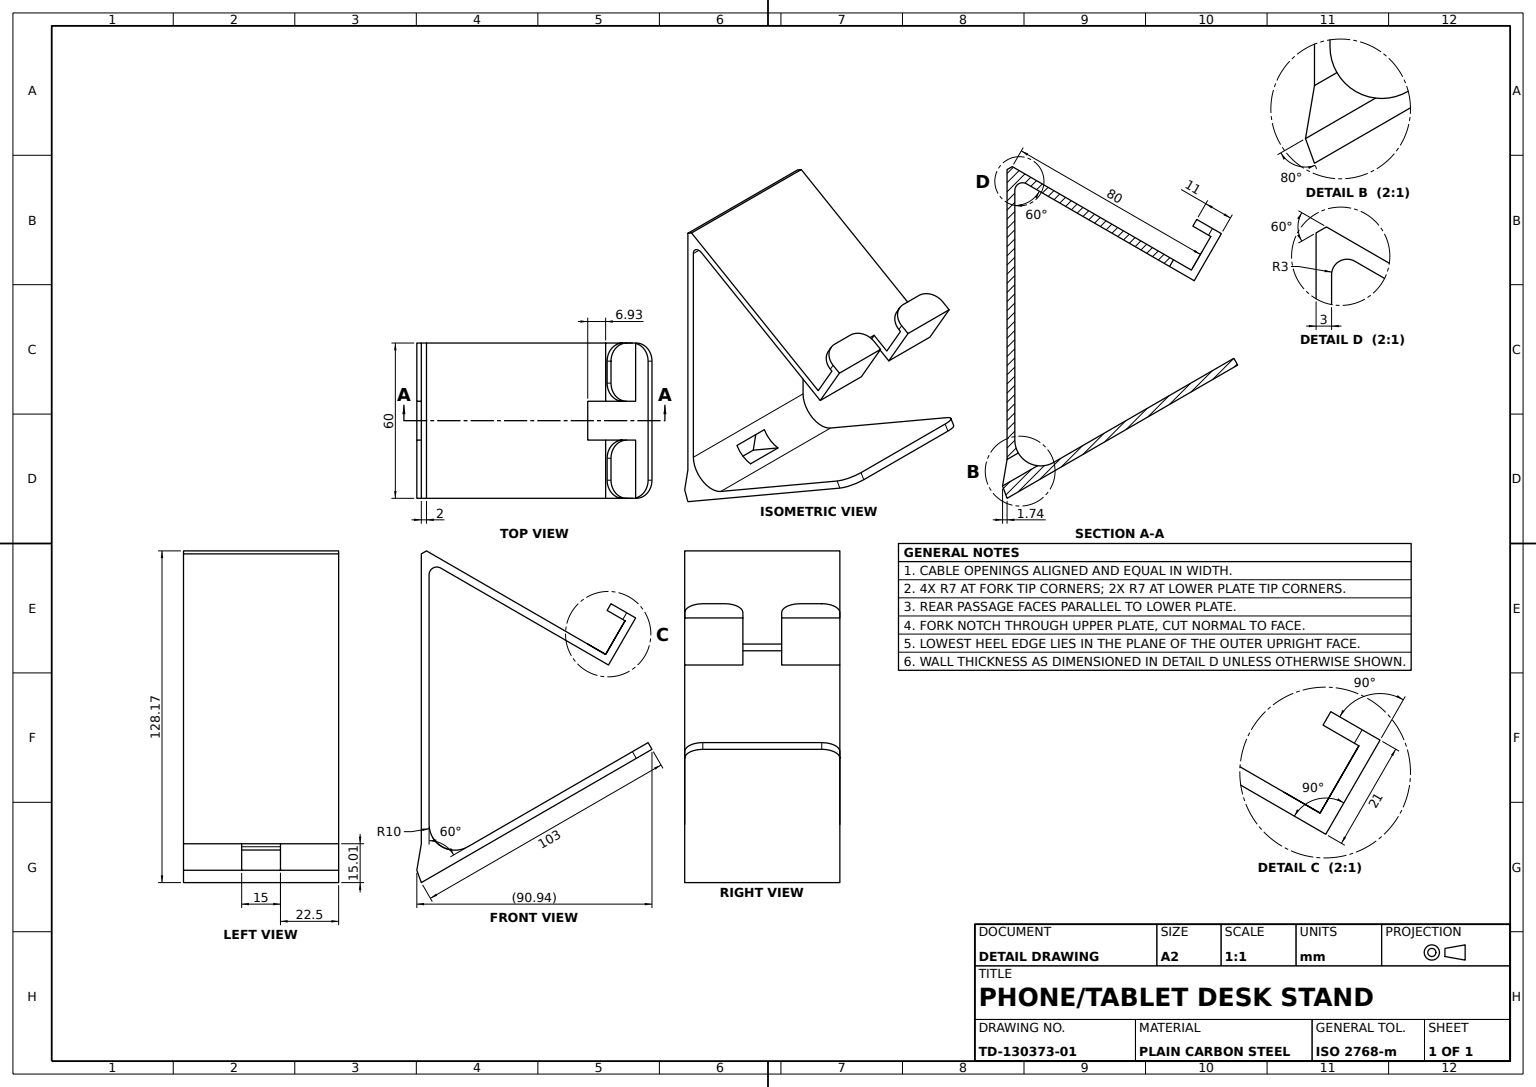
from build123d import *

# Parameters (mm, degrees)
STAND_BODY_60MM_DEPTH = 30
CABLE_NOTCH_SKETCH_W  = 15
CABLE_NOTCH_SKETCH_H  = 8
CABLE_NOTCH_DEPTH     = 152.518975709
SLOT_15X11_REACH      = 167.253
SLOT_15X11_SKETCH_W   = 15
SLOT_15X11_SKETCH_H   = 11
SLOT_EDGE_FILLET_R7_R = 7
BEND_FILLET_R7_R      = 7


with BuildPart() as part:
    # Stand Profile Sketch → Stand Body 60mm (new, symmetric)
    with BuildSketch(Plane.XY):
        with BuildLine():
            Line((0, 0), (80.483339502, 0))
            ThreePointArc((80.483339502, 0), (89.143593539, 5), (89.143593539, 15))
            Line((89.143593539, 15), (40.934846062, 98.5))
            ThreePointArc((40.934846062, 98.5), (38.336769851, 100), (35.738693639, 98.5))
            Line((35.738693639, 98.5), (-1.719854476, 33.619891486))
            Line((-1.719854476, 33.619891486), (-19.906387956, 44.119891486))
            Line((-19.906387956, 44.119891486), (-14.406387956, 53.646170928))
            Line((-14.406387956, 53.646170928), (-11.808311744, 52.146170928))
            Line((-11.808311744, 52.146170928), (-15.808311744, 45.217967697))
            Line((-15.808311744, 45.217967697), (-2.817930688, 37.717967697))
            Line((-2.817930688, 37.717967697), (37.182069312, 107))
            Line((37.182069312, 107), (39.491470389, 107))
            Line((39.491470389, 107), (95.494446501, 10))
            Line((95.494446501, 10), (102.118365096, 2))
            Line((102.118365096, 2), (103, -3))
            Line((103, -3), (0, -3))
            Line((0, -3), (0, 0))
        make_face()
    extrude(amount=STAND_BODY_60MM_DEPTH, both=True)

    # Cable Notch Sketch → Cable Notch (cut, through all)
    with BuildSketch(Plane(origin=(0, 0, 0), x_dir=(0, 0, -1), z_dir=(1, 0, 0))):
        with Locations((0, 6)):
            Rectangle(CABLE_NOTCH_SKETCH_W, CABLE_NOTCH_SKETCH_H)
    extrude(amount=CABLE_NOTCH_DEPTH, mode=Mode.SUBTRACT)

    # Slot 15x11 Sketch → Slot 15x11 (cut, up to next)
    with BuildSketch(Plane(origin=(-34.034264386, 19.649691705, 0), x_dir=(0, 0, 1), z_dir=(-0.8660254037844446, 0.49999999999998995, 0)), mode=Mode.PRIVATE) as slot_15x11_sk1:
        with Locations((0, 33.755752861)):
            Rectangle(SLOT_15X11_SKETCH_W, SLOT_15X11_SKETCH_H)
    slot_15x11_tool1 = extrude(slot_15x11_sk1.sketch, amount=-SLOT_15X11_REACH, mode=Mode.PRIVATE) & part.part
    add(slot_15x11_tool1.solids().sort_by_distance((-17.156388, 48.883031, 0))[0], mode=Mode.SUBTRACT)

    # Slot Edge Fillet R7
    slot_edge_fillet_r7_edges = [part.edges().sort_by_distance(p)[0] for p in [
        (-13.10734985, 52.896170928, -30),
        (-13.10734985, 52.896170928, 30),
        (-13.10734985, 52.896170928, 7.5),
        (-13.10734985, 52.896170928, -7.5),
    ]]
    fillet(slot_edge_fillet_r7_edges, radius=SLOT_EDGE_FILLET_R7_R)

    # Bend Fillet R7
    bend_fillet_r7_edges = [part.edges().sort_by_distance(p)[0] for p in [
        (0, -1.5, -30),
        (0, -1.5, 30),
    ]]
    fillet(bend_fillet_r7_edges, radius=BEND_FILLET_R7_R)


solid = part.part
